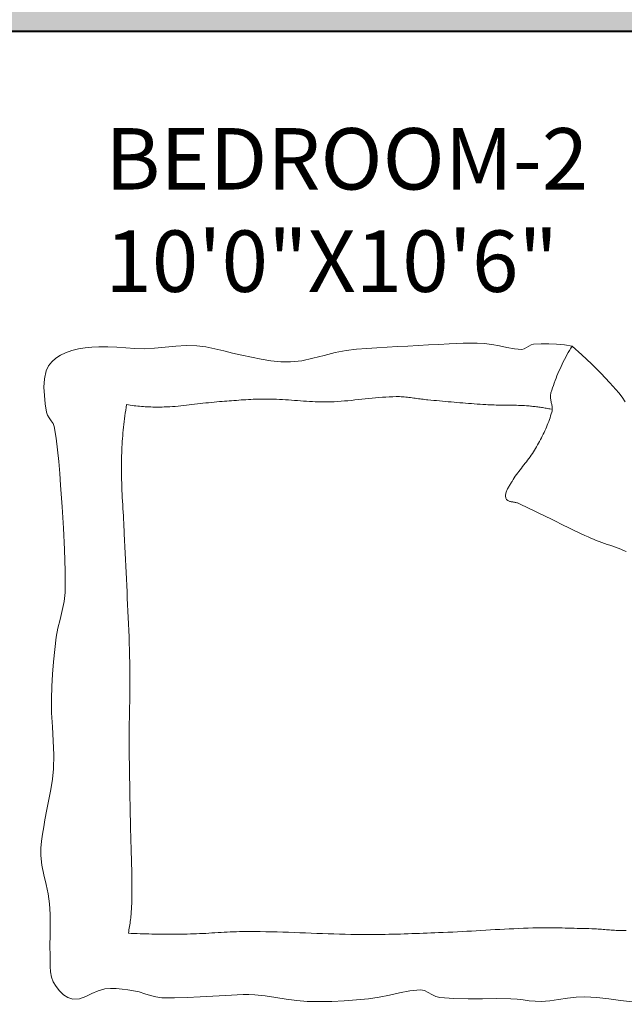
# Model space of a CAD drawing. Units: inches. Extents: x 1441 to 2460, y 1648 to 2683.
# Tile 15 of 35: x 1786 to 1845, y 2058 to 2154. Entities that reach past the tile are written whole.
import ezdxf

# ---------------------------------------------------------------- set-up
doc = ezdxf.new("R2010")
doc.units = ezdxf.units.IN
for name, color, linetype, lineweight in [('A-ANNO-DIMS', 2, 'Continuous', 18), ('A-AREA-IDEN', 7, 'Continuous', 20), ('A-FURN', 8, 'Continuous', 15), ('A-WALL', 7, 'Continuous', 40)]:
    doc.layers.add(name, color=color, linetype=linetype, lineweight=lineweight)
doc.layers.add('A-WALL-PATT', color=251, linetype='Continuous', lineweight=13, true_color=0x636466)
doc.styles.get("Standard").update_dxf_attribs({"font": 'arial.ttf'})
doc.dimstyles.get("Standard").update_dxf_attribs({"dimtxt": 0.18, "dimasz": 0.18, "dimexe": 0.18, "dimexo": 0.0625, "dimgap": 0.09, "dimtad": 0, "dimtih": 1, "dimtoh": 1, "dimdec": 4, "dimzin": 0, "dimdsep": 46, "dimtxsty": 'Standard', "dimcen": 0.09, "dimadec": 0, "dimazin": 0, "dimtfac": 1, "dimtdec": 4, "dimtofl": 0, "dimtmove": 0, "dimatfit": 3, "dimfxl": 1, "dimtolj": 1, "dimtzin": 0, "dimarcsym": 0})

# ---------------------------------------------------------------- blocks, each defined once
blk = doc.blocks.new('BED-DOUBLE-PLAN')
for p, q in [((64.222, 56.681), (64.382, 57.848)), ((5.285, 56.837), (4.851, 56.5)), ((5.748, 57.134), (5.285, 56.837)), ((20.15, 56.7), (20.254, 56.963)), ((20.254, 56.963), (20.361, 57.224)), ((57.398, 57.024), (57.394, 57.211)), ((57.399, 56.865), (57.398, 57.024)), ((57.398, 56.707), (57.399, 56.865)), ((4.851, 56.5), (3.888, 55.638)), ((19.761, 55.634), (19.856, 55.902)), ((19.856, 55.902), (19.952, 56.169)), ((19.952, 56.169), (20.05, 56.435)), ((20.05, 56.435), (20.15, 56.7)), ((57.353, 55.757), (57.363, 55.915)), ((57.363, 55.915), (57.373, 56.073)), ((57.373, 56.073), (57.382, 56.232)), ((57.382, 56.232), (57.389, 56.39)), ((57.389, 56.39), (57.394, 56.548)), ((57.394, 56.548), (57.398, 56.707)), ((64.06, 55.515), (64.222, 56.681)), ((3.888, 55.638), (2.949, 54.748)), ((19.474, 54.832), (19.571, 55.099)), ((19.571, 55.099), (19.666, 55.367)), ((19.666, 55.367), (19.761, 55.634)), ((57.279, 54.807), (57.291, 54.965)), ((57.291, 54.965), (57.304, 55.123)), ((57.304, 55.123), (57.316, 55.282)), ((57.316, 55.282), (57.329, 55.44)), ((57.329, 55.44), (57.341, 55.598)), ((57.341, 55.598), (57.353, 55.757)), ((63.929, 54.347), (64.06, 55.515)), ((2.949, 54.748), (2.036, 53.833)), ((19.059, 53.778), (19.169, 54.039)), ((19.169, 54.039), (19.274, 54.302)), ((19.274, 54.302), (19.375, 54.566)), ((19.375, 54.566), (19.474, 54.832)), ((57.227, 53.856), (57.232, 54.015)), ((57.232, 54.015), (57.239, 54.173)), ((57.239, 54.173), (57.247, 54.332)), ((57.247, 54.332), (57.257, 54.49)), ((57.257, 54.49), (57.268, 54.649)), ((57.268, 54.649), (57.279, 54.807)), ((63.863, 53.174), (63.929, 54.347)), ((2.036, 53.833), (1.148, 52.892)), ((18.629, 52.834), (18.788, 53.177)), ((18.788, 53.177), (18.945, 53.52)), ((18.945, 53.52), (19.059, 53.778)), ((57.194, 52.705), (57.202, 52.993)), ((57.202, 52.993), (57.21, 53.28)), ((57.21, 53.28), (57.218, 53.568)), ((57.218, 53.568), (57.227, 53.856)), ((63.897, 52.321), (63.863, 53.174)), ((1.148, 52.892), (0.288, 51.928)), ((18.143, 51.812), (18.306, 52.152)), ((18.306, 52.152), (18.468, 52.493)), ((18.468, 52.493), (18.629, 52.834)), ((57.171, 51.841), (57.178, 52.129)), ((57.178, 52.129), (57.186, 52.417)), ((57.186, 52.417), (57.194, 52.705)), ((64.002, 51.471), (63.897, 52.321)), ((0.178, 51.18), (0.104, 50.426)), ((0.288, 51.928), (0.178, 51.18)), ((0.288, 51.928), (0.502, 51.799)), ((0.502, 51.799), (0.719, 51.672)), ((0.719, 51.672), (0.936, 51.548)), ((0.936, 51.548), (1.156, 51.426)), ((1.156, 51.426), (1.377, 51.308)), ((1.377, 51.308), (1.6, 51.192)), ((1.6, 51.192), (1.824, 51.079)), ((1.824, 51.079), (2.05, 50.968)), ((17.648, 50.793), (17.814, 51.132)), ((17.814, 51.132), (17.979, 51.472)), ((17.979, 51.472), (18.143, 51.812)), ((57.152, 50.976), (57.158, 51.265)), ((57.158, 51.265), (57.164, 51.553)), ((57.164, 51.553), (57.171, 51.841)), ((64.135, 50.622), (64.002, 51.471)), ((0.104, 50.426), (0.065, 49.669)), ((2.05, 50.968), (2.277, 50.861)), ((2.277, 50.861), (2.505, 50.756)), ((2.505, 50.756), (2.735, 50.654)), ((2.735, 50.654), (2.966, 50.555)), ((2.966, 50.555), (3.198, 50.459)), ((3.198, 50.459), (3.432, 50.366)), ((3.432, 50.366), (3.666, 50.276)), ((3.666, 50.276), (3.901, 50.189)), ((3.901, 50.189), (4.138, 50.105)), ((4.138, 50.105), (4.375, 50.024)), ((17.147, 49.777), (17.314, 50.116)), ((17.314, 50.116), (17.481, 50.455)), ((17.481, 50.455), (17.648, 50.793)), ((57.138, 49.824), (57.14, 50.112)), ((57.14, 50.112), (57.143, 50.4)), ((57.143, 50.4), (57.147, 50.688)), ((57.147, 50.688), (57.152, 50.976)), ((64.256, 49.773), (64.135, 50.622)), ((0.065, 49.669), (0.062, 48.911)), ((4.375, 50.024), (4.613, 49.946)), ((4.613, 49.946), (4.852, 49.871)), ((4.852, 49.871), (4.943, 49.848)), ((4.943, 49.848), (5.034, 49.833)), ((5.034, 49.833), (5.127, 49.826)), ((5.127, 49.826), (5.22, 49.825)), ((5.22, 49.825), (5.314, 49.829)), ((5.314, 49.829), (5.409, 49.839)), ((5.409, 49.839), (5.504, 49.852)), ((5.504, 49.852), (5.6, 49.868)), ((5.6, 49.868), (5.695, 49.886)), ((5.695, 49.886), (5.791, 49.905)), ((5.791, 49.905), (5.887, 49.924)), ((5.887, 49.924), (5.983, 49.943)), ((5.983, 49.943), (6.079, 49.96)), ((6.079, 49.96), (6.174, 49.974)), ((6.174, 49.974), (6.269, 49.984)), ((6.269, 49.984), (6.363, 49.99)), ((6.326, 49.172), (6.307, 49.053)), ((6.347, 49.291), (6.326, 49.172)), ((6.368, 49.41), (6.347, 49.291)), ((6.363, 49.99), (6.457, 49.991)), ((6.39, 49.528), (6.368, 49.41)), ((6.412, 49.647), (6.39, 49.528)), ((6.436, 49.765), (6.412, 49.647)), ((6.46, 49.883), (6.436, 49.765)), ((6.457, 49.991), (6.55, 49.986)), ((6.55, 49.986), (6.643, 49.973)), ((6.643, 49.973), (6.734, 49.952)), ((6.734, 49.952), (6.921, 49.899)), ((6.921, 49.899), (7.107, 49.841)), ((7.107, 49.841), (7.292, 49.781)), ((7.292, 49.781), (7.476, 49.717)), ((7.476, 49.717), (7.659, 49.65)), ((7.659, 49.65), (7.841, 49.58)), ((7.841, 49.58), (8.022, 49.507)), ((8.022, 49.507), (8.202, 49.431)), ((8.202, 49.431), (8.381, 49.353)), ((8.381, 49.353), (8.56, 49.273)), ((8.56, 49.273), (8.737, 49.19)), ((8.737, 49.19), (8.913, 49.105)), ((8.913, 49.105), (9.088, 49.019)), ((16.647, 48.762), (16.813, 49.1)), ((16.813, 49.1), (16.98, 49.439)), ((16.98, 49.439), (17.147, 49.777)), ((57.137, 49.536), (57.138, 49.824)), ((57.137, 49.248), (57.137, 49.536)), ((57.139, 48.96), (57.137, 49.248)), ((64.322, 48.92), (64.256, 49.773)), ((0.062, 48.911), (0.095, 48.156)), ((0.095, 48.156), (0.161, 47.92)), ((6.193, 48.215), (6.18, 48.095)), ((6.207, 48.335), (6.193, 48.215)), ((6.221, 48.455), (6.207, 48.335)), ((6.237, 48.575), (6.221, 48.455)), ((6.253, 48.694), (6.237, 48.575)), ((6.27, 48.814), (6.253, 48.694)), ((6.288, 48.933), (6.27, 48.814)), ((6.307, 49.053), (6.288, 48.933)), ((9.088, 49.019), (9.263, 48.93)), ((9.263, 48.93), (9.436, 48.84)), ((9.436, 48.84), (9.609, 48.748)), ((9.609, 48.748), (9.781, 48.655)), ((9.781, 48.655), (9.952, 48.56)), ((9.952, 48.56), (10.122, 48.465)), ((10.122, 48.465), (10.291, 48.368)), ((10.291, 48.368), (10.462, 48.268)), ((10.462, 48.268), (10.629, 48.163)), ((10.629, 48.163), (10.794, 48.054)), ((16.315, 48.084), (16.481, 48.423)), ((16.481, 48.423), (16.647, 48.762)), ((57.142, 48.672), (57.139, 48.96)), ((57.147, 48.384), (57.142, 48.672)), ((57.153, 48.096), (57.147, 48.384)), ((64.258, 47.737), (64.311, 48.328)), ((64.311, 48.328), (64.322, 48.92)), ((0.161, 47.92), (0.294, 47.701)), ((0.294, 47.701), (0.446, 47.487)), ((0.446, 47.487), (0.571, 47.267)), ((0.571, 47.267), (0.62, 47.031)), ((6.114, 47.295), (6.104, 47.096)), ((6.127, 47.494), (6.114, 47.295)), ((6.136, 47.614), (6.127, 47.494)), ((6.146, 47.734), (6.136, 47.614)), ((6.156, 47.855), (6.146, 47.734)), ((6.168, 47.975), (6.156, 47.855)), ((6.18, 48.095), (6.168, 47.975)), ((10.794, 48.054), (10.957, 47.942)), ((10.957, 47.942), (11.118, 47.827)), ((11.118, 47.827), (11.277, 47.709)), ((11.277, 47.709), (11.435, 47.59)), ((11.435, 47.59), (11.593, 47.469)), ((11.593, 47.469), (11.749, 47.347)), ((11.749, 47.347), (11.905, 47.224)), ((11.905, 47.224), (12.061, 47.101)), ((15.824, 47.063), (15.987, 47.404)), ((15.987, 47.404), (16.151, 47.744)), ((16.151, 47.744), (16.315, 48.084)), ((57.167, 47.636), (57.153, 48.096)), ((57.182, 47.175), (57.167, 47.636)), ((57.2, 46.714), (57.182, 47.175)), ((64.117, 46.556), (64.185, 47.146)), ((64.185, 47.146), (64.258, 47.737)), ((0.562, 46.291), (0.434, 45.558)), ((0.62, 47.031), (0.562, 46.291)), ((6.076, 46.3), (6.072, 46.1)), ((6.081, 46.499), (6.076, 46.3)), ((6.087, 46.698), (6.081, 46.499)), ((6.095, 46.897), (6.087, 46.698)), ((6.104, 47.096), (6.095, 46.897)), ((12.061, 47.101), (12.218, 46.979)), ((12.218, 46.979), (12.374, 46.857)), ((12.374, 46.857), (12.532, 46.737)), ((12.532, 46.737), (12.691, 46.618)), ((12.691, 46.618), (12.851, 46.501)), ((12.851, 46.501), (13.012, 46.387)), ((13.012, 46.387), (13.176, 46.276)), ((13.176, 46.276), (13.342, 46.169)), ((15.527, 46.141), (15.539, 46.218)), ((15.539, 46.218), (15.551, 46.295)), ((15.551, 46.295), (15.564, 46.372)), ((15.564, 46.372), (15.578, 46.447)), ((15.578, 46.447), (15.595, 46.52)), ((15.595, 46.52), (15.614, 46.591)), ((15.614, 46.591), (15.636, 46.659)), ((15.636, 46.659), (15.663, 46.722)), ((15.663, 46.722), (15.824, 47.063)), ((57.22, 46.253), (57.2, 46.714)), ((57.241, 45.792), (57.22, 46.253)), ((64.074, 45.964), (64.117, 46.556)), ((0.434, 45.558), (0.277, 44.827)), ((6.062, 45.303), (6.06, 45.104)), ((6.064, 45.502), (6.062, 45.303)), ((6.067, 45.702), (6.064, 45.502)), ((6.069, 45.901), (6.067, 45.702)), ((6.072, 46.1), (6.069, 45.901)), ((13.342, 46.169), (13.511, 46.065)), ((13.511, 46.065), (13.587, 46.019)), ((13.587, 46.019), (13.664, 45.971)), ((13.664, 45.971), (13.742, 45.922)), ((13.742, 45.922), (13.822, 45.871)), ((13.822, 45.871), (13.902, 45.821)), ((13.902, 45.821), (13.983, 45.771)), ((13.983, 45.771), (14.065, 45.723)), ((14.065, 45.723), (14.147, 45.676)), ((14.147, 45.676), (14.231, 45.631)), ((14.231, 45.631), (14.314, 45.589)), ((14.314, 45.589), (14.398, 45.551)), ((14.398, 45.551), (14.483, 45.517)), ((14.483, 45.517), (14.567, 45.487)), ((14.567, 45.487), (14.652, 45.463)), ((14.652, 45.463), (14.737, 45.445)), ((14.737, 45.445), (14.822, 45.434)), ((14.822, 45.434), (14.907, 45.429)), ((14.907, 45.429), (14.992, 45.433)), ((14.992, 45.433), (15.076, 45.445)), ((15.076, 45.445), (15.16, 45.466)), ((15.16, 45.466), (15.221, 45.49)), ((15.221, 45.49), (15.274, 45.522)), ((15.274, 45.522), (15.32, 45.561)), ((15.32, 45.561), (15.36, 45.608)), ((15.36, 45.608), (15.394, 45.66)), ((15.394, 45.66), (15.423, 45.718)), ((15.423, 45.718), (15.448, 45.78)), ((15.448, 45.78), (15.468, 45.847)), ((15.468, 45.847), (15.486, 45.917)), ((15.486, 45.917), (15.502, 45.99)), ((15.502, 45.99), (15.515, 46.065)), ((15.515, 46.065), (15.527, 46.141)), ((57.264, 45.332), (57.241, 45.792)), ((57.289, 44.871), (57.264, 45.332)), ((64.052, 44.569), (64.074, 45.964)), ((0.277, 44.827), (0.13, 44.094)), ((6.045, 44.306), (6.039, 44.107)), ((6.05, 44.506), (6.045, 44.306)), ((6.054, 44.705), (6.05, 44.506)), ((6.057, 44.904), (6.054, 44.705)), ((6.06, 45.104), (6.057, 44.904)), ((57.314, 44.411), (57.289, 44.871)), ((57.34, 43.95), (57.314, 44.411)), ((64.063, 43.173), (64.052, 44.569)), ((0.035, 43.356), (0.002, 42.668)), ((0.13, 44.094), (0.035, 43.356)), ((6.011, 43.51), (5.993, 43.227)), ((6.022, 43.709), (6.011, 43.51)), ((6.031, 43.908), (6.022, 43.709)), ((6.039, 44.107), (6.031, 43.908)), ((57.367, 43.49), (57.34, 43.95)), ((57.394, 43.029), (57.367, 43.49)), ((0.002, 42.668), (0.002, 41.978)), ((5.935, 42.376), (5.914, 42.093)), ((5.955, 42.66), (5.935, 42.376)), ((5.975, 42.943), (5.955, 42.66)), ((5.993, 43.227), (5.975, 42.943)), ((57.42, 42.569), (57.394, 43.029)), ((57.447, 42.108), (57.42, 42.569)), ((64.074, 41.778), (64.063, 43.173)), ((0.002, 41.978), (0.023, 41.288)), ((5.869, 41.527), (5.846, 41.243)), ((5.892, 41.81), (5.869, 41.527)), ((5.914, 42.093), (5.892, 41.81)), ((57.474, 41.648), (57.447, 42.108)), ((57.499, 41.187), (57.474, 41.648)), ((64.051, 40.384), (64.074, 41.778)), ((0.023, 41.288), (0.053, 40.599)), ((0.053, 40.599), (0.083, 39.909)), ((5.798, 40.677), (5.774, 40.394)), ((5.822, 40.96), (5.798, 40.677)), ((5.846, 41.243), (5.822, 40.96)), ((57.524, 40.727), (57.499, 41.187)), ((57.548, 40.266), (57.524, 40.727)), ((0.083, 39.909), (0.124, 38.9)), ((5.698, 39.545), (5.673, 39.262)), ((5.724, 39.828), (5.698, 39.545)), ((5.749, 40.111), (5.724, 39.828)), ((5.774, 40.394), (5.749, 40.111)), ((57.57, 39.806), (57.548, 40.266)), ((57.59, 39.345), (57.57, 39.806)), ((63.96, 38.994), (64.051, 40.384)), ((0.124, 38.9), (0.172, 37.892)), ((5.621, 38.696), (5.596, 38.413)), ((5.647, 38.979), (5.621, 38.696)), ((5.673, 39.262), (5.647, 38.979)), ((57.609, 38.884), (57.59, 39.345)), ((57.623, 38.511), (57.609, 38.884)), ((57.637, 38.138), (57.623, 38.511)), ((63.663, 38.235), (63.855, 38.605)), ((63.855, 38.605), (63.96, 38.994)), ((0.172, 37.892), (0.227, 36.884)), ((5.513, 37.537), (5.494, 37.382)), ((5.53, 37.692), (5.513, 37.537)), ((5.545, 37.847), (5.53, 37.692)), ((5.57, 38.13), (5.545, 37.847)), ((5.596, 38.413), (5.57, 38.13)), ((57.652, 37.765), (57.637, 38.138)), ((57.666, 37.393), (57.652, 37.765)), ((63.274, 37.501), (63.447, 37.871)), ((63.447, 37.871), (63.663, 38.235)), ((0.227, 36.884), (0.286, 35.876)), ((5.388, 36.608), (5.366, 36.454)), ((5.41, 36.763), (5.388, 36.608)), ((5.432, 36.918), (5.41, 36.763)), ((5.453, 37.073), (5.432, 36.918)), ((5.474, 37.227), (5.453, 37.073)), ((5.494, 37.382), (5.474, 37.227)), ((57.68, 37.02), (57.666, 37.393)), ((57.693, 36.647), (57.68, 37.02)), ((57.706, 36.274), (57.693, 36.647)), ((63.206, 37.11), (63.274, 37.501)), ((63.291, 36.09), (63.206, 37.11)), ((0.286, 35.876), (0.348, 34.868)), ((5.27, 35.679), (5.256, 35.524)), ((5.287, 35.834), (5.27, 35.679)), ((5.304, 35.989), (5.287, 35.834)), ((5.324, 36.144), (5.304, 35.989)), ((5.344, 36.299), (5.324, 36.144)), ((5.366, 36.454), (5.344, 36.299)), ((57.718, 35.901), (57.706, 36.274)), ((57.73, 35.528), (57.718, 35.901)), ((63.474, 35.079), (63.291, 36.09)), ((0.348, 34.868), (0.404, 33.866)), ((5.23, 35.059), (5.228, 34.903)), ((5.228, 34.903), (5.229, 34.747)), ((5.229, 34.747), (5.239, 34.409)), ((5.236, 35.214), (5.23, 35.059)), ((5.245, 35.369), (5.236, 35.214)), ((5.256, 35.524), (5.245, 35.369)), ((57.741, 35.155), (57.73, 35.528)), ((57.751, 34.782), (57.741, 35.155)), ((57.761, 34.409), (57.751, 34.782)), ((63.703, 34.073), (63.474, 35.079)), ((0.404, 33.866), (0.456, 32.863)), ((5.239, 34.409), (5.254, 34.072)), ((5.254, 34.072), (5.274, 33.735)), ((5.274, 33.735), (5.297, 33.397)), ((57.769, 34.036), (57.761, 34.409)), ((57.776, 33.663), (57.769, 34.036)), ((63.921, 33.064), (63.703, 34.073)), ((0.456, 32.863), (0.516, 31.861)), ((5.297, 33.397), (5.324, 33.06)), ((5.324, 33.06), (5.354, 32.724)), ((5.354, 32.724), (5.386, 32.387)), ((57.782, 33.29), (57.776, 33.663)), ((57.787, 32.917), (57.782, 33.29)), ((57.79, 32.543), (57.787, 32.917)), ((64.075, 32.048), (63.921, 33.064)), ((0.516, 31.861), (0.599, 30.861)), ((5.386, 32.387), (5.42, 32.05)), ((5.42, 32.05), (5.455, 31.714)), ((57.792, 32.17), (57.79, 32.543)), ((57.79, 31.424), (57.792, 31.797)), ((57.792, 31.797), (57.792, 32.17)), ((64.186, 30.851), (64.075, 32.048)), ((0.599, 30.861), (0.719, 29.866)), ((5.455, 31.714), (5.491, 31.377)), ((5.491, 31.377), (5.526, 31.04)), ((5.526, 31.04), (5.561, 30.704)), ((57.777, 30.314), (57.785, 30.869)), ((57.785, 30.869), (57.79, 31.424)), ((64.273, 29.652), (64.186, 30.851)), ((0.719, 29.866), (0.929, 28.772)), ((5.561, 30.704), (5.595, 30.367)), ((5.595, 30.367), (5.627, 30.03)), ((5.627, 30.03), (5.656, 29.694)), ((57.765, 29.759), (57.777, 30.314)), ((5.656, 29.694), (5.683, 29.357)), ((5.683, 29.357), (5.706, 29.019)), ((5.706, 29.019), (5.725, 28.682)), ((57.735, 28.65), (57.751, 29.204)), ((57.751, 29.204), (57.765, 29.759)), ((64.329, 28.45), (64.273, 29.652)), ((0.929, 28.772), (1.205, 27.689)), ((5.725, 28.682), (5.74, 28.344)), ((5.74, 28.344), (5.749, 28.007)), ((5.749, 28.007), (5.752, 27.715)), ((57.698, 27.54), (57.718, 28.095)), ((57.718, 28.095), (57.735, 28.65)), ((64.349, 27.249), (64.329, 28.45)), ((1.205, 27.689), (1.489, 26.608)), ((5.744, 27.131), (5.734, 26.839)), ((5.75, 27.423), (5.744, 27.131)), ((5.752, 27.715), (5.75, 27.423)), ((57.657, 26.431), (57.678, 26.985)), ((57.678, 26.985), (57.698, 27.54)), ((64.328, 26.047), (64.349, 27.249)), ((1.489, 26.608), (1.722, 25.521)), ((5.704, 26.255), (5.686, 25.964)), ((5.72, 26.547), (5.704, 26.255)), ((5.734, 26.839), (5.72, 26.547)), ((57.636, 25.876), (57.657, 26.431)), ((64.248, 25.017), (64.328, 26.047)), ((1.722, 25.521), (1.846, 24.419)), ((5.622, 25.089), (5.6, 24.797)), ((5.644, 25.38), (5.622, 25.089)), ((5.666, 25.672), (5.644, 25.38)), ((5.686, 25.964), (5.666, 25.672)), ((57.595, 24.766), (57.615, 25.321)), ((57.615, 25.321), (57.636, 25.876)), ((64.106, 23.991), (64.248, 25.017)), ((1.846, 24.419), (1.831, 23.458)), ((5.556, 24.214), (5.535, 23.922)), ((5.577, 24.505), (5.556, 24.214)), ((5.6, 24.797), (5.577, 24.505)), ((57.556, 23.657), (57.575, 24.212)), ((57.575, 24.212), (57.595, 24.766)), ((1.831, 23.458), (1.723, 22.5)), ((5.499, 23.338), (5.485, 23.047)), ((5.516, 23.63), (5.499, 23.338)), ((5.535, 23.922), (5.516, 23.63)), ((57.525, 22.547), (57.54, 23.102)), ((57.54, 23.102), (57.556, 23.657)), ((63.939, 22.967), (64.106, 23.991)), ((1.723, 22.5), (1.555, 21.544)), ((5.467, 22.463), (5.464, 22.171)), ((5.464, 22.171), (5.465, 21.936)), ((5.475, 22.755), (5.467, 22.463)), ((5.485, 23.047), (5.475, 22.755)), ((57.512, 21.992), (57.525, 22.547)), ((63.782, 21.942), (63.939, 22.967)), ((1.555, 21.544), (1.362, 20.592)), ((5.465, 21.936), (5.467, 21.701)), ((5.467, 21.701), (5.472, 21.467)), ((5.472, 21.467), (5.478, 21.232)), ((5.478, 21.232), (5.486, 20.998)), ((57.495, 20.882), (57.502, 21.437)), ((57.502, 21.437), (57.512, 21.992)), ((63.671, 20.913), (63.782, 21.942)), ((1.362, 20.592), (1.181, 19.64)), ((5.486, 20.998), (5.495, 20.763)), ((5.495, 20.763), (5.506, 20.529)), ((5.506, 20.529), (5.518, 20.295)), ((5.518, 20.295), (5.531, 20.06)), ((57.492, 20.327), (57.495, 20.882)), ((57.493, 20.027), (57.492, 20.327)), ((63.649, 20.346), (63.671, 20.913)), ((63.657, 19.777), (63.649, 20.346)), ((1.181, 19.64), (0.996, 18.76)), ((5.531, 20.06), (5.546, 19.826)), ((5.546, 19.826), (5.561, 19.592)), ((5.561, 19.592), (5.577, 19.358)), ((5.577, 19.358), (5.594, 19.123)), ((57.497, 19.727), (57.493, 20.027)), ((57.504, 19.427), (57.497, 19.727)), ((57.513, 19.127), (57.504, 19.427)), ((63.683, 19.209), (63.657, 19.777)), ((0.996, 18.76), (0.773, 17.887)), ((5.594, 19.123), (5.612, 18.889)), ((5.612, 18.889), (5.629, 18.655)), ((5.629, 18.655), (5.647, 18.421)), ((5.647, 18.421), (5.666, 18.187)), ((57.525, 18.827), (57.513, 19.127)), ((57.538, 18.527), (57.525, 18.827)), ((57.554, 18.227), (57.538, 18.527)), ((63.715, 18.64), (63.683, 19.209)), ((63.74, 18.071), (63.715, 18.64)), ((0.773, 17.887), (0.551, 17.013)), ((5.666, 18.187), (5.684, 17.953)), ((5.684, 17.953), (5.702, 17.719)), ((5.702, 17.719), (5.721, 17.485)), ((5.721, 17.485), (5.743, 17.213)), ((57.57, 17.927), (57.554, 18.227)), ((57.587, 17.627), (57.57, 17.927)), ((57.605, 17.327), (57.587, 17.627)), ((57.623, 17.027), (57.605, 17.327)), ((63.8, 16.821), (63.74, 18.071)), ((0.551, 17.013), (0.366, 16.135)), ((5.743, 17.213), (5.768, 16.942)), ((5.768, 16.942), (5.794, 16.671)), ((5.794, 16.671), (5.823, 16.399)), ((5.823, 16.399), (5.853, 16.128)), ((57.641, 16.727), (57.623, 17.027)), ((57.659, 16.427), (57.641, 16.727)), ((57.676, 16.127), (57.659, 16.427)), ((63.878, 15.571), (63.8, 16.821)), ((0.366, 16.135), (0.257, 15.246)), ((5.853, 16.128), (5.884, 15.857)), ((5.884, 15.857), (5.916, 15.587)), ((5.916, 15.587), (5.948, 15.316)), ((57.692, 15.827), (57.676, 16.127)), ((57.706, 15.527), (57.692, 15.827)), ((57.719, 15.227), (57.706, 15.527)), ((63.95, 14.321), (63.878, 15.571)), ((0.257, 15.246), (0.244, 14.217)), ((5.948, 15.316), (5.981, 15.045)), ((5.981, 15.045), (6.013, 14.774)), ((6.013, 14.774), (6.044, 14.503)), ((6.044, 14.503), (6.075, 14.232)), ((57.73, 14.927), (57.719, 15.227)), ((57.739, 14.627), (57.73, 14.927)), ((57.745, 14.327), (57.739, 14.627)), ((0.244, 14.217), (0.31, 13.189)), ((6.075, 14.232), (6.104, 13.961)), ((6.104, 13.961), (6.131, 13.69)), ((6.131, 13.69), (6.157, 13.419)), ((57.749, 14.039), (57.745, 14.327)), ((57.752, 13.751), (57.749, 14.039)), ((57.754, 13.463), (57.752, 13.751)), ((63.987, 13.071), (63.95, 14.321)), ((0.31, 13.189), (0.413, 12.16)), ((6.157, 13.419), (6.18, 13.147)), ((6.18, 13.147), (6.201, 12.876)), ((6.201, 12.876), (6.219, 12.604)), ((6.219, 12.604), (6.233, 12.332)), ((57.756, 13.174), (57.754, 13.463)), ((57.757, 12.886), (57.756, 13.174)), ((57.756, 12.31), (57.757, 12.598)), ((57.757, 12.598), (57.757, 12.886)), ((63.964, 11.821), (63.987, 13.071)), ((0.413, 12.16), (0.51, 11.13)), ((6.233, 12.332), (6.244, 12.06)), ((6.244, 12.06), (6.249, 11.876)), ((6.249, 11.876), (6.252, 11.692)), ((6.252, 11.692), (6.254, 11.508)), ((57.749, 11.446), (57.752, 11.734)), ((57.752, 11.734), (57.754, 12.022)), ((57.754, 12.022), (57.756, 12.31)), ((63.889, 11.262), (63.964, 11.821)), ((0.51, 11.13), (0.56, 10.1)), ((6.235, 10.588), (6.226, 10.405)), ((6.242, 10.772), (6.235, 10.588)), ((6.248, 10.956), (6.242, 10.772)), ((6.251, 11.14), (6.248, 10.956)), ((6.253, 11.324), (6.251, 11.14)), ((6.254, 11.508), (6.253, 11.324)), ((57.734, 10.582), (57.74, 10.87)), ((57.74, 10.87), (57.744, 11.158)), ((57.744, 11.158), (57.749, 11.446)), ((63.572, 10.169), (63.745, 10.713)), ((63.745, 10.713), (63.889, 11.262)), ((0.56, 10.1), (0.539, 9.213)), ((6.173, 9.67), (6.155, 9.487)), ((6.189, 9.854), (6.173, 9.67)), ((6.203, 10.037), (6.189, 9.854)), ((6.215, 10.221), (6.203, 10.037)), ((6.226, 10.405), (6.215, 10.221)), ((57.703, 9.43), (57.712, 9.718)), ((57.712, 9.718), (57.72, 10.006)), ((57.72, 10.006), (57.727, 10.294)), ((57.727, 10.294), (57.734, 10.582)), ((63.284, 9.068), (63.406, 9.622)), ((63.406, 9.622), (63.572, 10.169)), ((0.539, 9.213), (0.478, 8.327)), ((6.067, 8.756), (6.041, 8.575)), ((6.092, 8.939), (6.067, 8.756)), ((6.115, 9.121), (6.092, 8.939)), ((6.136, 9.304), (6.115, 9.121)), ((6.155, 9.487), (6.136, 9.304)), ((29.335, 8.65), (29.964, 8.67)), ((29.964, 8.67), (30.594, 8.689)), ((30.594, 8.689), (31.224, 8.705)), ((31.224, 8.705), (31.613, 8.712)), ((31.613, 8.712), (32.002, 8.718)), ((32.002, 8.718), (32.391, 8.72)), ((32.391, 8.72), (32.781, 8.721)), ((32.781, 8.721), (33.17, 8.72)), ((33.17, 8.72), (33.559, 8.717)), ((33.559, 8.717), (33.948, 8.713)), ((33.948, 8.713), (34.338, 8.707)), ((34.338, 8.707), (34.727, 8.701)), ((34.727, 8.701), (35.116, 8.694)), ((35.116, 8.694), (35.506, 8.687)), ((35.506, 8.687), (35.895, 8.679)), ((35.895, 8.679), (36.284, 8.672)), ((36.284, 8.672), (36.674, 8.665)), ((36.674, 8.665), (37.063, 8.659)), ((37.063, 8.659), (37.452, 8.653)), ((40.601, 8.658), (40.999, 8.663)), ((40.999, 8.663), (41.397, 8.668)), ((41.397, 8.668), (41.795, 8.674)), ((41.795, 8.674), (42.193, 8.68)), ((42.193, 8.68), (42.591, 8.687)), ((42.591, 8.687), (42.989, 8.694)), ((42.989, 8.694), (43.387, 8.701)), ((43.387, 8.701), (43.785, 8.708)), ((43.785, 8.708), (44.183, 8.716)), ((44.183, 8.716), (44.581, 8.723)), ((44.581, 8.723), (44.979, 8.731)), ((44.979, 8.731), (45.376, 8.739)), ((45.376, 8.739), (45.774, 8.746)), ((45.774, 8.746), (46.172, 8.754)), ((46.172, 8.754), (46.57, 8.761)), ((46.57, 8.761), (46.968, 8.768)), ((46.968, 8.768), (47.336, 8.775)), ((47.336, 8.775), (47.704, 8.784)), ((47.704, 8.784), (48.071, 8.793)), ((48.071, 8.793), (48.439, 8.804)), ((48.439, 8.804), (48.807, 8.815)), ((48.807, 8.815), (49.174, 8.827)), ((49.174, 8.827), (49.542, 8.839)), ((49.542, 8.839), (49.91, 8.85)), ((49.91, 8.85), (50.278, 8.862)), ((50.278, 8.862), (50.645, 8.873)), ((50.645, 8.873), (51.013, 8.884)), ((51.013, 8.884), (51.381, 8.893)), ((51.381, 8.893), (51.748, 8.902)), ((51.748, 8.902), (52.116, 8.909)), ((52.116, 8.909), (52.484, 8.915)), ((52.484, 8.915), (52.851, 8.919)), ((52.851, 8.919), (53.219, 8.92)), ((53.219, 8.92), (53.587, 8.92)), ((53.587, 8.92), (53.955, 8.917)), ((53.955, 8.917), (54.322, 8.912)), ((54.322, 8.912), (54.491, 8.908)), ((54.491, 8.908), (54.659, 8.902)), ((54.659, 8.902), (54.827, 8.896)), ((54.827, 8.896), (54.996, 8.888)), ((54.996, 8.888), (55.164, 8.878)), ((55.164, 8.878), (55.332, 8.867)), ((55.332, 8.867), (55.5, 8.855)), ((55.5, 8.855), (55.668, 8.841)), ((55.668, 8.841), (55.836, 8.826)), ((55.836, 8.826), (56.004, 8.809)), ((56.004, 8.809), (56.172, 8.791)), ((56.172, 8.791), (56.339, 8.772)), ((56.339, 8.772), (56.507, 8.751)), ((56.507, 8.751), (56.674, 8.729)), ((56.674, 8.729), (56.841, 8.705)), ((56.841, 8.705), (57.008, 8.68)), ((57.008, 8.68), (57.174, 8.654)), ((57.672, 8.567), (57.683, 8.855)), ((57.683, 8.855), (57.694, 9.142)), ((57.694, 9.142), (57.703, 9.43)), ((63.198, 8.508), (63.284, 9.068)), ((0.478, 8.327), (0.407, 7.441)), ((6.041, 8.575), (6.013, 8.393)), ((6.013, 8.393), (6.289, 8.349)), ((6.289, 8.349), (6.564, 8.306)), ((6.564, 8.306), (6.841, 8.266)), ((6.841, 8.266), (7.117, 8.228)), ((7.117, 8.228), (7.394, 8.191)), ((7.394, 8.191), (7.671, 8.157)), ((7.671, 8.157), (7.949, 8.125)), ((7.949, 8.125), (8.226, 8.094)), ((8.226, 8.094), (8.504, 8.066)), ((8.504, 8.066), (8.783, 8.04)), ((8.783, 8.04), (9.061, 8.016)), ((9.061, 8.016), (9.339, 7.993)), ((9.339, 7.993), (9.618, 7.973)), ((9.618, 7.973), (9.897, 7.955)), ((9.897, 7.955), (10.175, 7.939)), ((10.175, 7.939), (10.454, 7.925)), ((10.454, 7.925), (10.733, 7.913)), ((10.733, 7.913), (11.012, 7.903)), ((11.012, 7.903), (11.291, 7.894)), ((11.291, 7.894), (11.57, 7.888)), ((11.57, 7.888), (11.924, 7.884)), ((11.924, 7.884), (12.277, 7.883)), ((12.277, 7.883), (12.631, 7.886)), ((12.631, 7.886), (12.984, 7.892)), ((12.984, 7.892), (13.338, 7.9)), ((13.338, 7.9), (13.691, 7.912)), ((13.691, 7.912), (14.044, 7.925)), ((14.044, 7.925), (14.397, 7.94)), ((14.397, 7.94), (14.751, 7.957)), ((14.751, 7.957), (15.104, 7.975)), ((15.104, 7.975), (15.457, 7.995)), ((15.457, 7.995), (15.811, 8.015)), ((15.811, 8.015), (16.164, 8.035)), ((16.164, 8.035), (16.517, 8.056)), ((16.517, 8.056), (16.87, 8.076)), ((16.87, 8.076), (17.224, 8.097)), ((17.224, 8.097), (17.577, 8.116)), ((17.577, 8.116), (17.93, 8.134)), ((17.93, 8.134), (18.283, 8.152)), ((18.283, 8.152), (18.637, 8.167)), ((18.637, 8.167), (19.266, 8.194)), ((19.266, 8.194), (19.895, 8.222)), ((19.895, 8.222), (20.525, 8.251)), ((20.525, 8.251), (21.154, 8.28)), ((21.154, 8.28), (21.783, 8.311)), ((21.783, 8.311), (22.412, 8.341)), ((22.412, 8.341), (23.042, 8.372)), ((23.042, 8.372), (23.671, 8.403)), ((23.671, 8.403), (24.3, 8.434)), ((24.3, 8.434), (24.929, 8.464)), ((24.929, 8.464), (25.559, 8.494)), ((25.559, 8.494), (26.188, 8.523)), ((26.188, 8.523), (26.817, 8.551)), ((26.817, 8.551), (27.447, 8.578)), ((27.447, 8.578), (28.076, 8.604)), ((28.076, 8.604), (28.705, 8.628)), ((28.705, 8.628), (29.335, 8.65)), ((37.452, 8.653), (37.841, 8.649)), ((37.841, 8.649), (38.231, 8.646)), ((38.231, 8.646), (38.62, 8.645)), ((38.62, 8.645), (39.009, 8.645)), ((39.009, 8.645), (39.407, 8.647)), ((39.407, 8.647), (39.805, 8.65)), ((39.805, 8.65), (40.203, 8.654)), ((40.203, 8.654), (40.601, 8.658)), ((57.174, 8.654), (57.34, 8.626)), ((57.34, 8.626), (57.506, 8.597)), ((57.506, 8.597), (57.672, 8.567)), ((63.071, 7.38), (63.122, 7.945)), ((63.122, 7.945), (63.198, 8.508)), ((0.407, 7.441), (0.359, 6.555)), ((63.06, 6.816), (63.071, 7.38)), ((63.104, 6.255), (63.06, 6.816)), ((0.359, 6.555), (0.366, 5.67)), ((63.28, 5.623), (63.104, 6.255)), ((0.366, 5.67), (0.403, 5.005)), ((0.403, 5.005), (0.461, 4.337)), ((63.563, 5.008), (63.28, 5.623)), ((63.859, 4.399), (63.563, 5.008)), ((0.461, 4.337), (0.559, 3.676)), ((64.071, 3.785), (63.859, 4.399)), ((0.559, 3.676), (0.713, 3.032)), ((0.713, 3.032), (0.943, 2.414)), ((63.955, 2.665), (64.104, 3.152)), ((64.104, 3.152), (64.071, 3.785)), ((0.943, 2.414), (1.182, 1.944)), ((1.182, 1.944), (1.477, 1.491)), ((12.738, 1.867), (13.892, 1.947)), ((13.892, 1.947), (15.985, 2.09)), ((15.985, 2.09), (18.08, 2.228)), ((18.08, 2.228), (20.175, 2.338)), ((20.175, 2.338), (22.271, 2.396)), ((22.271, 2.396), (24.367, 2.38)), ((24.367, 2.38), (25.251, 2.29)), ((25.251, 2.29), (26.124, 2.109)), ((26.124, 2.109), (26.993, 1.884)), ((63.298, 1.834), (63.674, 2.224)), ((63.674, 2.224), (63.955, 2.665)), ((1.477, 1.491), (1.827, 1.085)), ((1.827, 1.085), (2.233, 0.757)), ((7.317, 0.83), (7.582, 1.025)), ((7.582, 1.025), (7.854, 1.201)), ((7.854, 1.201), (8.149, 1.31)), ((8.149, 1.31), (9.288, 1.504)), ((9.288, 1.504), (10.434, 1.655)), ((10.434, 1.655), (11.585, 1.773)), ((11.585, 1.773), (12.738, 1.867)), ((26.993, 1.884), (27.863, 1.668)), ((27.863, 1.668), (28.742, 1.509)), ((28.742, 1.509), (29.941, 1.367)), ((29.941, 1.367), (31.143, 1.249)), ((31.143, 1.249), (32.348, 1.156)), ((32.348, 1.156), (33.554, 1.09)), ((33.554, 1.09), (34.76, 1.051)), ((34.76, 1.051), (36.132, 1.067)), ((36.132, 1.067), (37.503, 1.138)), ((37.503, 1.138), (38.874, 1.222)), ((38.874, 1.222), (40.245, 1.275)), ((40.245, 1.275), (41.615, 1.254)), ((41.615, 1.254), (42.615, 1.155)), ((42.615, 1.155), (43.607, 0.99)), ((43.607, 0.99), (44.596, 0.79)), ((61.444, 0.958), (61.942, 1.046)), ((61.942, 1.046), (62.409, 1.227)), ((62.409, 1.227), (62.864, 1.5)), ((62.864, 1.5), (63.298, 1.834)), ((2.233, 0.757), (2.695, 0.537)), ((2.695, 0.537), (3.482, 0.364)), ((3.482, 0.364), (4.291, 0.315)), ((4.291, 0.315), (5.113, 0.355)), ((5.113, 0.355), (5.935, 0.45)), ((5.935, 0.45), (6.746, 0.564)), ((6.746, 0.564), (7.043, 0.661)), ((7.043, 0.661), (7.317, 0.83)), ((44.596, 0.79), (45.584, 0.588)), ((45.584, 0.588), (46.576, 0.415)), ((46.576, 0.415), (47.273, 0.3)), ((47.273, 0.3), (47.97, 0.177)), ((47.97, 0.177), (48.668, 0.07)), ((48.668, 0.07), (49.368, 0.004)), ((49.368, 0.004), (50.07, 0.002)), ((50.07, 0.002), (51.018, 0.111)), ((51.018, 0.111), (51.957, 0.3)), ((51.957, 0.3), (52.892, 0.521)), ((52.892, 0.521), (53.83, 0.725)), ((53.83, 0.725), (54.776, 0.863)), ((54.776, 0.863), (55.797, 0.922)), ((55.797, 0.922), (56.82, 0.927)), ((56.82, 0.927), (57.845, 0.908)), ((57.845, 0.908), (58.869, 0.895)), ((58.869, 0.895), (59.893, 0.917)), ((59.893, 0.917), (60.407, 0.926)), ((60.407, 0.926), (60.928, 0.929)), ((60.928, 0.929), (61.444, 0.958))]:
    blk.add_line(p, q)
blk = doc.blocks.new('*D67')
at = {"layer": 'A-ANNO-DIMS', "color": 0, "lineweight": -2, "transparency": 16777216}
for p, q in [((1889.448, 2298.695), (1916.216, 2298.695)), ((1916.036, 2298.515), (1916.036, 2055.938)), ((1916.036, 1812.997), (1916.036, 2055.574)), ((1758.224, 1812.817), (1916.216, 1812.817))]:
    blk.add_line(p, q, dxfattribs=at)
at = {"layer": 'A-ANNO-DIMS', "color": 0, "transparency": 16777216}
for points in [[(1916.006, 2298.515), (1916.066, 2298.515), (1916.036, 2298.695)], [(1916.006, 1812.997), (1916.066, 1812.997), (1916.036, 1812.817)]]:
    blk.add_solid(points, dxfattribs=at)
at = {"layer": 'Defpoints', "color": 0, "transparency": 16777216}
for p in [(1889.386, 2298.695), (1916.036, 2298.695), (1758.161, 1812.817)]:
    blk.add_point(p, dxfattribs=at)
at = {"layer": 'A-ANNO-DIMS', "color": 0, "transparency": 16777216, "insert": (1916.036, 2055.756), "char_height": 0.18, "attachment_point": 5}
blk.add_mtext('\\A1;485.9', dxfattribs=at)

msp = doc.modelspace()

# ---------------------------------------------------------------- hatches: boundary and pattern name
at = {"layer": 'A-WALL-PATT'}
h = msp.add_hatch(color=256, dxfattribs=at)
h.dxf.hatch_style = 1
h.paths.add_polyline_path([(1627.5085, 2298.6952), (1568.8859, 2298.6952), (1568.8859, 2246.9605), (1577.8859, 2246.9605), (1577.8859, 2289.6952), (1627.5085, 2289.6952), (1627.5085, 2294.1952)])
h.paths.add_polyline_path([(1675.5777, 2298.6952), (1651.5085, 2298.6952), (1651.5085, 2289.6952), (1675.5777, 2289.6952), (1675.5777, 2294.1952)])
h.paths.add_polyline_path([(1667.3859, 2289.6952), (1662.8859, 2289.6952), (1662.8859, 2233.0622), (1667.3859, 2233.0622)])
h.paths.add_polyline_path([(1715.8721, 2294.3362), (1715.8721, 2295.2788), (1715.8721, 2298.6952), (1699.5777, 2298.6952), (1699.5777, 2289.6952), (1715.8721, 2289.6952)])
h.paths.add_polyline_path([(1707.8859, 2289.6952), (1703.3859, 2289.6952), (1703.3859, 2199.6952), (1707.8859, 2199.6952)])
h.paths.add_polyline_path([(1760.3859, 2204.637), (1755.8859, 2204.637), (1755.8859, 2199.6952), (1667.3859, 2199.6952), (1667.3859, 2204.637), (1662.8859, 2204.637), (1662.8859, 2195.1952), (1760.3859, 2195.1952)])
h.paths.add_polyline_path([(1760.3859, 2289.6952), (1755.8859, 2289.6952), (1755.8859, 2233.0622), (1760.3859, 2233.0622)])
h.paths.add_polyline_path([(1889.3859, 2298.6952), (1739.8721, 2298.6952), (1739.8721, 2289.6952), (1880.3859, 2289.6952), (1880.3859, 2250.8051), (1889.3859, 2250.8051)])
h.paths.add_polyline_path([(1889.3859, 2202.8051), (1880.3859, 2202.8051), (1880.3859, 2157.6952), (1747.948, 2157.6952), (1747.948, 2153.1952), (1755.8859, 2153.1952), (1755.8859, 2058.005), (1760.3859, 2058.005), (1760.3859, 2153.1952), (1880.3859, 2153.1952), (1880.3859, 2124.108), (1889.3859, 2124.108)])
h.paths.add_polyline_path([(1889.3859, 1984.8305), (1880.3859, 1984.8305), (1880.3859, 1834.1952), (1889.3859, 1834.1952)])
h.paths.add_polyline_path([(1889.3859, 2076.108), (1880.3859, 2076.108), (1880.3859, 2008.8305), (1889.3859, 2008.8305)])
h.paths.add_polyline_path([(1880.3859, 2027.1952), (1800.8859, 2027.1952), (1800.8859, 2000.9452), (1805.3859, 2000.9452), (1805.3859, 2022.6952), (1880.3859, 2022.6952)])
h.paths.add_polyline_path([(1800.8859, 2027.1952), (1760.3859, 2027.1952), (1760.3859, 2030.7912), (1755.8859, 2030.7912), (1755.8859, 2022.6952), (1800.8859, 2022.6952)])
h.paths.add_polyline_path([(1880.3859, 1974.6952), (1805.3859, 1974.6952), (1805.3859, 1978.7973), (1800.8859, 1978.7973), (1800.8859, 1974.6952), (1794.8823, 1974.6952), (1794.8823, 1970.1952), (1800.8859, 1970.1952), (1805.3859, 1970.1952), (1880.3859, 1970.1952)])
h.paths.add_polyline_path([(1760.3859, 1974.6952), (1755.8859, 1974.6952), (1755.8859, 1925.6952), (1751.8616, 1925.6952), (1751.8616, 1921.1952), (1760.3859, 1921.1952)])
h.paths.add_polyline_path([(1760.3859, 1921.1952), (1755.8859, 1921.1952), (1755.8859, 1843.1952), (1760.3859, 1843.1952)])
h.paths.add_polyline_path([(1799.1136, 1838.6952), (1799.1136, 1843.1952), (1760.3859, 1843.1952), (1751.8944, 1843.1952), (1751.8944, 1834.1952), (1758.1615, 1834.1952), (1799.1136, 1834.1952)])
h.paths.add_polyline_path([(1880.3859, 1843.1952), (1859.1136, 1843.1952), (1859.1136, 1834.1952), (1880.3859, 1834.1952)])
h.paths.add_polyline_path([(1577.8859, 1857.7914), (1568.8859, 1857.7914), (1568.8859, 1834.1952), (1695.0034, 1834.1952), (1695.0034, 1838.6952), (1695.0034, 1843.1952), (1577.8859, 1843.1952)])
h.paths.add_polyline_path([(1577.8859, 1959.2399), (1573.3859, 1959.2399), (1568.8859, 1959.2399), (1568.8859, 1905.7914), (1577.8859, 1905.7914), (1577.8859, 1921.1952), (1703.3859, 1921.1952), (1707.8859, 1921.1952), (1715.1501, 1921.1952), (1715.1501, 1925.6952), (1707.8859, 1925.6952), (1703.3859, 1925.6952), (1577.8859, 1925.6952)])
h.paths.add_polyline_path([(1577.8859, 2106.6907), (1568.8859, 2106.6907), (1568.8859, 2019.2399), (1577.8859, 2019.2399)])
h.paths.add_polyline_path([(1707.8859, 2051.6952), (1703.3859, 2051.6952), (1703.3859, 2048.6952), (1703.3859, 1925.6952), (1707.8859, 1925.6952)])
h.paths.add_polyline_path([(1703.3859, 2051.6952), (1676.3859, 2051.6952), (1676.3859, 2048.6952), (1703.3859, 2048.6952)])
h.paths.add_polyline_path([(1703.3859, 2102.6952), (1676.3859, 2102.6952), (1676.3859, 2099.6952), (1685.3859, 2099.6952), (1703.3859, 2099.6952)])
h.paths.add_polyline_path([(1707.8859, 2153.1952), (1710.5611, 2153.1952), (1710.5611, 2157.6952), (1707.8859, 2157.6952), (1707.8859, 2195.1952), (1703.3859, 2195.1952), (1703.3859, 2099.6952), (1707.8859, 2099.6952)])
h.paths.add_polyline_path([(1577.8859, 2198.9605), (1568.8859, 2198.9605), (1568.8859, 2166.6907), (1577.8859, 2166.6907)])

# ---------------------------------------------------------------- linework, layer by layer
at = {"layer": 'A-WALL'}
msp.add_line((1760.3859, 2153.1952), (1880.3859, 2153.1952), dxfattribs=at)

# ---------------------------------------------------------------- block references
at = {"layer": 'A-FURN', "rotation": 270}
msp.add_blockref('BED-DOUBLE-PLAN', (1788.0907, 2122.7206), dxfattribs=at)

# ---------------------------------------------------------------- texts
at = {"layer": 'A-AREA-IDEN', "insert": (1794.4038, 2143.7255), "char_height": 6, "attachment_point": 1}
msp.add_mtext_dynamic_manual_height_columns('BEDROOM-2\\P10\'0"X10\'6"', width=85.554017, gutter_width=12.5, heights=[0], dxfattribs=at)

# ---------------------------------------------------------------- dimensions: what is measured, and where the dimension line sits
at = {"layer": 'A-ANNO-DIMS'}
dim = msp.add_linear_dim(base=(1916.0359, 2298.6952), p1=(1758.1615, 1812.8171), p2=(1889.3859, 2298.6952), angle=90, dimstyle='Standard', override={"dimdec": 1, "dimlfac": 1, "dimrnd": 0, "dimzin": 0, "dimdsep": 46, "dimlunit": 2}, dxfattribs=at)
dim.commit()
dim.dimension.update_dxf_attribs({"geometry": '*D67', "text_midpoint": (1916.0359, 2055.7561)})

doc.saveas('drawing.dxf')
